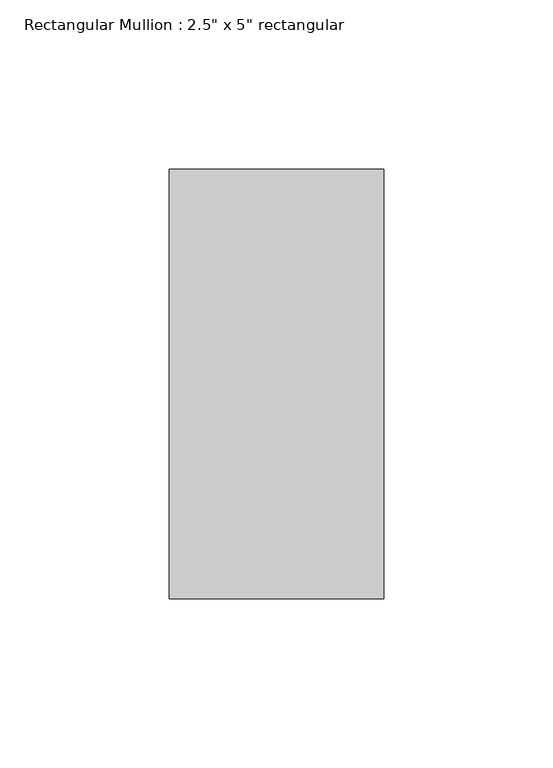
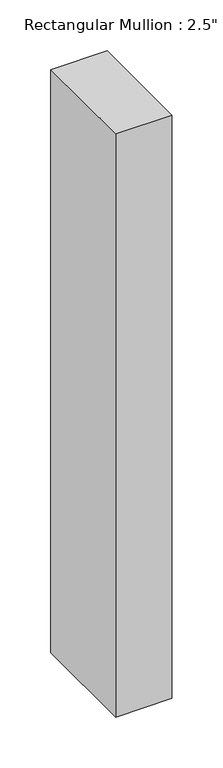
"""IFC4 building model written with IfcOpenShell, lengths in millimetres: member geometry."""

from ifc_helpers import new_model, si_unit, frame, origin, place, context, project, spatial, polyline, outline, extrude, source, transform, mapped, element, save


def member_c7c5a8a0(model_context):
    return source(origin(), model_context, "Body", "SweptSolid", [
        extrude(outline(polyline([(31.75, 63.5), (31.75, -63.5), (-31.75, -63.5), (-31.75, 63.5), (31.75, 63.5)])), frame((0.0, 0.0, -698.5), z_axis=(0.0, 0.0, 1.0), x_axis=(1.0, 0.0, 0.0)), (0.0, 0.0, 1.0), 698.5),
    ])


if __name__ == "__main__":
    model = new_model("IFC4")
    model_context = context("Model", 3, world=origin())
    ifc_project = project(units=[si_unit("LENGTHUNIT", "METRE", prefix="MILLI")], contexts=[model_context])
    site = spatial("IfcSite", under=ifc_project)
    building = spatial("IfcBuilding", under=site)
    placement = place(None, origin())
    member_shape = member_c7c5a8a0(model_context)
    element("IfcMember", 1, ObjectType="Rectangular Mullion : 2.5\" x 5\" rectangular", at=placement, inside=building, context=model_context, shape_type="MappedRepresentation", body=[
        mapped(member_shape, transform((0.0, 0.0, 0.0), x_axis=(1.0, 0.0, 0.0), y_axis=(0.0, 1.0, 0.0), z_axis=(0.0, 0.0, 1.0))),
    ])
    save(model, "model.ifc")

# Revit data of these elements
# Type "Rectangular Mullion : 2.5\" x 5\" rectangular"
#   built-in parameter 1007304 = 0.416667 (stored number, unit not read)
#   built-in parameter 1007301 = 0.104167 (stored number, unit not read)
#   built-in parameter 1007300 = 0.104167 (stored number, unit not read)
# Element 1 (IfcMember, "Rectangular Mullion : 2.5\" x 5\" rectangular")
#   Materials on its faces: "Aluminum"
# Materials
#   "Aluminum": class "Metal", colour RGB 247 247 247, transparency 0, Description = "Aluminum 6061", Cost = 0
